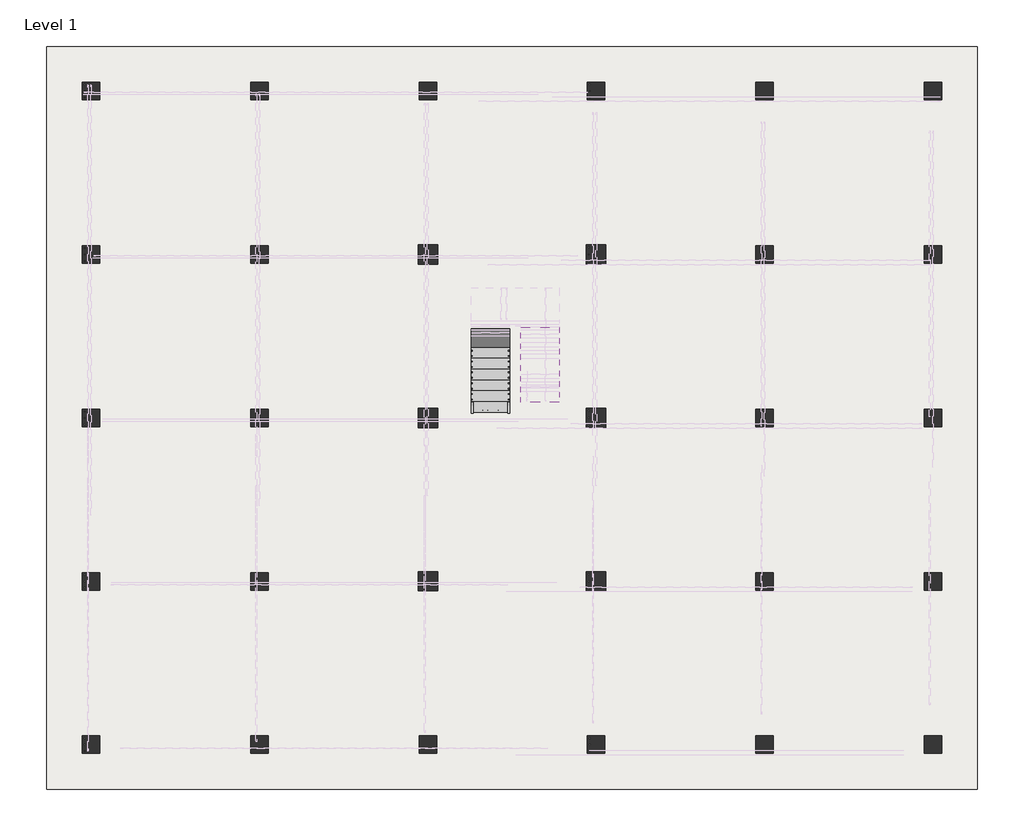
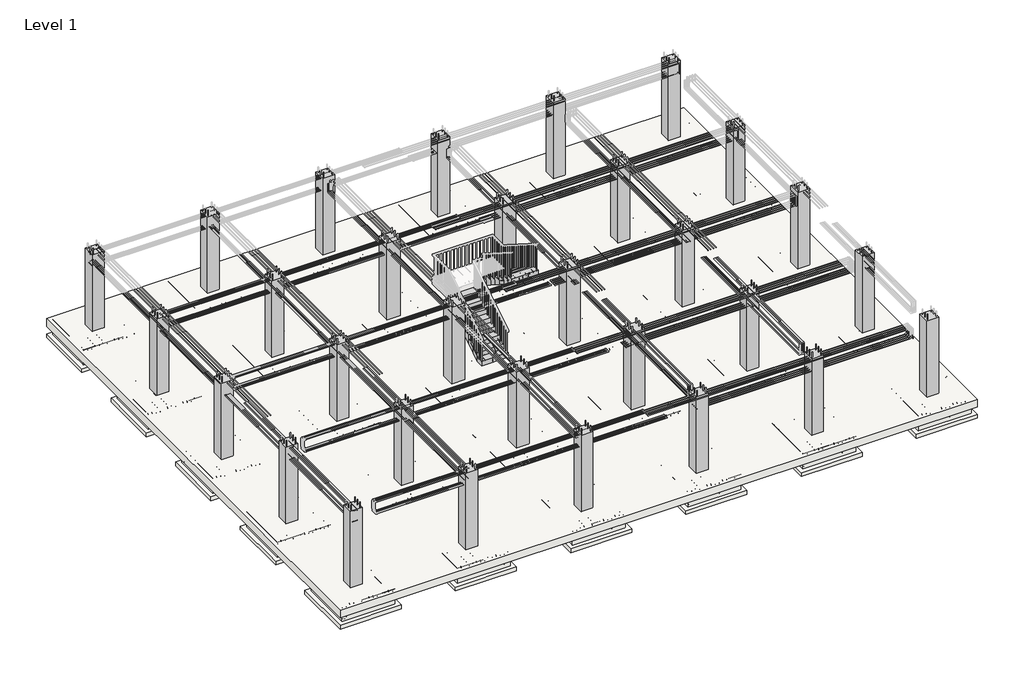
# One storey, part 1 of 17: 31 slabs, 30 columns, 2 stair flights.
"""IFC4 building model written with IfcOpenShell, lengths in millimetres."""

from ifc_helpers import new_model, si_unit, frame, origin, origin_with_axes, place, context, project, spatial, polyline, outline, extrude, faceted_brep, transform, mapped, element, save
from components import m_footing_rectangular_2000x2000x600_e4767d7a, m_footing_rectangular_2200x2200x650_5a9dd948

model = new_model("IFC4")

# Units and contexts
model_context = context("Model", 3, world=origin())
ifc_project = project(units=[si_unit("LENGTHUNIT", "METRE", prefix="MILLI")], contexts=[model_context])

# Site, building, storey
site = spatial("IfcSite", under=ifc_project)
building = spatial("IfcBuilding", under=site)
storey = spatial("IfcBuildingStorey", under=building, Name="Level 1", Elevation=0.0)

# Columns
placement = place(None, origin())
element("IfcColumn", 1, ObjectType="M_Concrete-Rectangular-Column : 450x450", at=placement, inside=storey, context=model_context, shape_type="SweptSolid", body=[
    extrude(outline(polyline([(-12509.3632003, 12560.009457), (-12509.3632003, 12110.009457), (-12959.3632003, 12110.009457), (-12959.3632003, 12560.009457), (-12509.3632003, 12560.009457)])), origin_with_axes(), (0.0, 0.0, 1.0), 3048.0),
])
element("IfcColumn", 2, ObjectType="M_Concrete-Rectangular-Column : 450x450", at=placement, inside=storey, context=model_context, shape_type="SweptSolid", body=[
    extrude(outline(polyline([(-8164.3632003, 12560.009457), (-8164.3632003, 12110.009457), (-8614.3632003, 12110.009457), (-8614.3632003, 12560.009457), (-8164.3632003, 12560.009457)])), origin_with_axes(), (0.0, 0.0, 1.0), 3048.0),
])
element("IfcColumn", 3, ObjectType="M_Concrete-Rectangular-Column : 450x450", at=placement, inside=storey, context=model_context, shape_type="SweptSolid", body=[
    extrude(outline(polyline([(-3819.3632003, 12560.009457), (-3819.3632003, 12110.009457), (-4269.3632003, 12110.009457), (-4269.3632003, 12560.009457), (-3819.3632003, 12560.009457)])), origin_with_axes(), (0.0, 0.0, 1.0), 3048.0),
])
element("IfcColumn", 4, ObjectType="M_Concrete-Rectangular-Column : 450x450", at=placement, inside=storey, context=model_context, shape_type="SweptSolid", body=[
    extrude(outline(polyline([(525.6367997, 12560.009457), (525.6367997, 12110.009457), (75.6367997, 12110.009457), (75.6367997, 12560.009457), (525.6367997, 12560.009457)])), origin_with_axes(), (0.0, 0.0, 1.0), 3048.0),
])
element("IfcColumn", 5, ObjectType="M_Concrete-Rectangular-Column : 450x450", at=placement, inside=storey, context=model_context, shape_type="SweptSolid", body=[
    extrude(outline(polyline([(4870.6367997, 12560.009457), (4870.6367997, 12110.009457), (4420.6367997, 12110.009457), (4420.6367997, 12560.009457), (4870.6367997, 12560.009457)])), origin_with_axes(), (0.0, 0.0, 1.0), 3048.0),
])
element("IfcColumn", 6, ObjectType="M_Concrete-Rectangular-Column : 450x450", at=placement, inside=storey, context=model_context, shape_type="SweptSolid", body=[
    extrude(outline(polyline([(9215.6367997, 12560.009457), (9215.6367997, 12110.009457), (8765.6367997, 12110.009457), (8765.6367997, 12560.009457), (9215.6367997, 12560.009457)])), origin_with_axes(), (0.0, 0.0, 1.0), 3048.0),
])
element("IfcColumn", 7, ObjectType="M_Concrete-Rectangular-Column : 450x450", at=placement, inside=storey, context=model_context, shape_type="SweptSolid", body=[
    extrude(outline(polyline([(-12509.3632003, 8343.009457), (-12509.3632003, 7893.009457), (-12959.3632003, 7893.009457), (-12959.3632003, 8343.009457), (-12509.3632003, 8343.009457)])), origin_with_axes(), (0.0, 0.0, 1.0), 3048.0),
])
element("IfcColumn", 8, ObjectType="M_Concrete-Rectangular-Column : 450x450", at=placement, inside=storey, context=model_context, shape_type="SweptSolid", body=[
    extrude(outline(polyline([(-8164.3632003, 8343.009457), (-8164.3632003, 7893.009457), (-8614.3632003, 7893.009457), (-8614.3632003, 8343.009457), (-8164.3632003, 8343.009457)])), origin_with_axes(), (0.0, 0.0, 1.0), 3048.0),
])
element("IfcColumn", 9, ObjectType="M_Concrete-Rectangular-Column : 450x450", at=placement, inside=storey, context=model_context, shape_type="SweptSolid", body=[
    extrude(outline(polyline([(4870.6367997, 8343.009457), (4870.6367997, 7893.009457), (4420.6367997, 7893.009457), (4420.6367997, 8343.009457), (4870.6367997, 8343.009457)])), origin_with_axes(), (0.0, 0.0, 1.0), 3048.0),
])
element("IfcColumn", 10, ObjectType="M_Concrete-Rectangular-Column : 450x450", at=placement, inside=storey, context=model_context, shape_type="SweptSolid", body=[
    extrude(outline(polyline([(9215.6367997, 8343.009457), (9215.6367997, 7893.009457), (8765.6367997, 7893.009457), (8765.6367997, 8343.009457), (9215.6367997, 8343.009457)])), origin_with_axes(), (0.0, 0.0, 1.0), 3048.0),
])
element("IfcColumn", 11, ObjectType="M_Concrete-Rectangular-Column : 450x450", at=placement, inside=storey, context=model_context, shape_type="SweptSolid", body=[
    extrude(outline(polyline([(-12509.3632003, 4126.009457), (-12509.3632003, 3676.009457), (-12959.3632003, 3676.009457), (-12959.3632003, 4126.009457), (-12509.3632003, 4126.009457)])), origin_with_axes(), (0.0, 0.0, 1.0), 3048.0),
])
element("IfcColumn", 12, ObjectType="M_Concrete-Rectangular-Column : 450x450", at=placement, inside=storey, context=model_context, shape_type="SweptSolid", body=[
    extrude(outline(polyline([(-8164.3632003, 4126.009457), (-8164.3632003, 3676.009457), (-8614.3632003, 3676.009457), (-8614.3632003, 4126.009457), (-8164.3632003, 4126.009457)])), origin_with_axes(), (0.0, 0.0, 1.0), 3048.0),
])
element("IfcColumn", 13, ObjectType="M_Concrete-Rectangular-Column : 450x450", at=placement, inside=storey, context=model_context, shape_type="SweptSolid", body=[
    extrude(outline(polyline([(4870.6367997, 4126.009457), (4870.6367997, 3676.009457), (4420.6367997, 3676.009457), (4420.6367997, 4126.009457), (4870.6367997, 4126.009457)])), origin_with_axes(), (0.0, 0.0, 1.0), 3048.0),
])
element("IfcColumn", 14, ObjectType="M_Concrete-Rectangular-Column : 450x450", at=placement, inside=storey, context=model_context, shape_type="SweptSolid", body=[
    extrude(outline(polyline([(9215.6367997, 4126.009457), (9215.6367997, 3676.009457), (8765.6367997, 3676.009457), (8765.6367997, 4126.009457), (9215.6367997, 4126.009457)])), origin_with_axes(), (0.0, 0.0, 1.0), 3048.0),
])
element("IfcColumn", 15, ObjectType="M_Concrete-Rectangular-Column : 450x450", at=placement, inside=storey, context=model_context, shape_type="SweptSolid", body=[
    extrude(outline(polyline([(-12509.3632003, -90.990543), (-12509.3632003, -540.990543), (-12959.3632003, -540.990543), (-12959.3632003, -90.990543), (-12509.3632003, -90.990543)])), origin_with_axes(), (0.0, 0.0, 1.0), 3048.0),
])
element("IfcColumn", 16, ObjectType="M_Concrete-Rectangular-Column : 450x450", at=placement, inside=storey, context=model_context, shape_type="SweptSolid", body=[
    extrude(outline(polyline([(-8164.3632003, -90.990543), (-8164.3632003, -540.990543), (-8614.3632003, -540.990543), (-8614.3632003, -90.990543), (-8164.3632003, -90.990543)])), origin_with_axes(), (0.0, 0.0, 1.0), 3048.0),
])
element("IfcColumn", 17, ObjectType="M_Concrete-Rectangular-Column : 450x450", at=placement, inside=storey, context=model_context, shape_type="SweptSolid", body=[
    extrude(outline(polyline([(4870.6367997, -90.990543), (4870.6367997, -540.990543), (4420.6367997, -540.990543), (4420.6367997, -90.990543), (4870.6367997, -90.990543)])), origin_with_axes(), (0.0, 0.0, 1.0), 3048.0),
])
element("IfcColumn", 18, ObjectType="M_Concrete-Rectangular-Column : 450x450", at=placement, inside=storey, context=model_context, shape_type="SweptSolid", body=[
    extrude(outline(polyline([(9215.6367997, -90.990543), (9215.6367997, -540.990543), (8765.6367997, -540.990543), (8765.6367997, -90.990543), (9215.6367997, -90.990543)])), origin_with_axes(), (0.0, 0.0, 1.0), 3048.0),
])
element("IfcColumn", 19, ObjectType="M_Concrete-Rectangular-Column : 450x450", at=placement, inside=storey, context=model_context, shape_type="SweptSolid", body=[
    extrude(outline(polyline([(-12509.3632003, -4307.990543), (-12509.3632003, -4757.990543), (-12959.3632003, -4757.990543), (-12959.3632003, -4307.990543), (-12509.3632003, -4307.990543)])), origin_with_axes(), (0.0, 0.0, 1.0), 3048.0),
])
element("IfcColumn", 20, ObjectType="M_Concrete-Rectangular-Column : 450x450", at=placement, inside=storey, context=model_context, shape_type="SweptSolid", body=[
    extrude(outline(polyline([(-8164.3632003, -4307.990543), (-8164.3632003, -4757.990543), (-8614.3632003, -4757.990543), (-8614.3632003, -4307.990543), (-8164.3632003, -4307.990543)])), origin_with_axes(), (0.0, 0.0, 1.0), 3048.0),
])
element("IfcColumn", 21, ObjectType="M_Concrete-Rectangular-Column : 450x450", at=placement, inside=storey, context=model_context, shape_type="SweptSolid", body=[
    extrude(outline(polyline([(-3819.3632003, -4307.990543), (-3819.3632003, -4757.990543), (-4269.3632003, -4757.990543), (-4269.3632003, -4307.990543), (-3819.3632003, -4307.990543)])), origin_with_axes(), (0.0, 0.0, 1.0), 3048.0),
])
element("IfcColumn", 22, ObjectType="M_Concrete-Rectangular-Column : 450x450", at=placement, inside=storey, context=model_context, shape_type="SweptSolid", body=[
    extrude(outline(polyline([(525.6367997, -4307.990543), (525.6367997, -4757.990543), (75.6367997, -4757.990543), (75.6367997, -4307.990543), (525.6367997, -4307.990543)])), origin_with_axes(), (0.0, 0.0, 1.0), 3048.0),
])
element("IfcColumn", 23, ObjectType="M_Concrete-Rectangular-Column : 450x450", at=placement, inside=storey, context=model_context, shape_type="SweptSolid", body=[
    extrude(outline(polyline([(4870.6367997, -4307.990543), (4870.6367997, -4757.990543), (4420.6367997, -4757.990543), (4420.6367997, -4307.990543), (4870.6367997, -4307.990543)])), origin_with_axes(), (0.0, 0.0, 1.0), 3048.0),
])
element("IfcColumn", 24, ObjectType="M_Concrete-Rectangular-Column : 450x450", at=placement, inside=storey, context=model_context, shape_type="SweptSolid", body=[
    extrude(outline(polyline([(9215.6367997, -4307.990543), (9215.6367997, -4757.990543), (8765.6367997, -4757.990543), (8765.6367997, -4307.990543), (9215.6367997, -4307.990543)])), origin_with_axes(), (0.0, 0.0, 1.0), 3048.0),
])
element("IfcColumn", 25, ObjectType="M_Concrete-Rectangular-Column : 500x500", at=placement, inside=storey, context=model_context, shape_type="SweptSolid", body=[
    extrude(outline(polyline([(-3794.3632003, 8368.009457), (-3794.3632003, 7868.009457), (-4294.3632003, 7868.009457), (-4294.3632003, 8368.009457), (-3794.3632003, 8368.009457)])), origin_with_axes(), (0.0, 0.0, 1.0), 3048.0),
])
element("IfcColumn", 26, ObjectType="M_Concrete-Rectangular-Column : 500x500", at=placement, inside=storey, context=model_context, shape_type="SweptSolid", body=[
    extrude(outline(polyline([(550.6367997, 8368.009457), (550.6367997, 7868.009457), (50.6367997, 7868.009457), (50.6367997, 8368.009457), (550.6367997, 8368.009457)])), origin_with_axes(), (0.0, 0.0, 1.0), 3048.0),
])
element("IfcColumn", 27, ObjectType="M_Concrete-Rectangular-Column : 500x500", at=placement, inside=storey, context=model_context, shape_type="SweptSolid", body=[
    extrude(outline(polyline([(550.6367997, 4151.009457), (550.6367997, 3651.009457), (50.6367997, 3651.009457), (50.6367997, 4151.009457), (550.6367997, 4151.009457)])), origin_with_axes(), (0.0, 0.0, 1.0), 3048.0),
])
element("IfcColumn", 28, ObjectType="M_Concrete-Rectangular-Column : 500x500", at=placement, inside=storey, context=model_context, shape_type="SweptSolid", body=[
    extrude(outline(polyline([(-3794.3632003, 4151.009457), (-3794.3632003, 3651.009457), (-4294.3632003, 3651.009457), (-4294.3632003, 4151.009457), (-3794.3632003, 4151.009457)])), origin_with_axes(), (0.0, 0.0, 1.0), 3048.0),
])
element("IfcColumn", 29, ObjectType="M_Concrete-Rectangular-Column : 500x500", at=placement, inside=storey, context=model_context, shape_type="SweptSolid", body=[
    extrude(outline(polyline([(-3794.3632003, -65.990543), (-3794.3632003, -565.990543), (-4294.3632003, -565.990543), (-4294.3632003, -65.990543), (-3794.3632003, -65.990543)])), origin_with_axes(), (0.0, 0.0, 1.0), 3048.0),
])
element("IfcColumn", 30, ObjectType="M_Concrete-Rectangular-Column : 500x500", at=placement, inside=storey, context=model_context, shape_type="SweptSolid", body=[
    extrude(outline(polyline([(550.6367997, -65.990543), (550.6367997, -565.990543), (50.6367997, -565.990543), (50.6367997, -65.990543), (550.6367997, -65.990543)])), origin_with_axes(), (0.0, 0.0, 1.0), 3048.0),
])

# Slabs
element("IfcSlab", 31, ObjectType="Generic 300mm", at=placement, inside=storey, context=model_context, shape_type="SweptSolid", body=[
    extrude(outline(polyline([(10140.6367997, 13485.009457), (10140.6367997, -5682.990543), (-13884.3632003, -5682.990543), (-13884.3632003, 13485.009457), (10140.6367997, 13485.009457)])), frame((0.0, 0.0, -300.0), z_axis=(0.0, 0.0, 1.0), x_axis=(1.0, 0.0, 0.0)), (0.0, 0.0, 1.0), 300.0),
])
m_footing_rectangular_2000x2000x600_shape = m_footing_rectangular_2000x2000x600_e4767d7a(model_context)
element("IfcSlab", 32, ObjectType="M_Footing-Rectangular : 2000x2000x600", at=placement, inside=storey, context=model_context, shape_type="MappedRepresentation", body=[
    mapped(m_footing_rectangular_2000x2000x600_shape, transform((-12734.3632003, 12335.009457, 0.0), x_axis=(1.0, 0.0, 0.0), y_axis=(0.0, 1.0, 0.0), z_axis=(0.0, 0.0, 1.0))),
])
element("IfcSlab", 33, ObjectType="M_Footing-Rectangular : 2000x2000x600", at=placement, inside=storey, context=model_context, shape_type="MappedRepresentation", body=[
    mapped(m_footing_rectangular_2000x2000x600_shape, transform((-8389.3632003, 12335.009457, 0.0), x_axis=(1.0, 0.0, 0.0), y_axis=(0.0, 1.0, 0.0), z_axis=(0.0, 0.0, 1.0))),
])
element("IfcSlab", 34, ObjectType="M_Footing-Rectangular : 2000x2000x600", at=placement, inside=storey, context=model_context, shape_type="MappedRepresentation", body=[
    mapped(m_footing_rectangular_2000x2000x600_shape, transform((-4044.3632003, 12335.009457, 0.0), x_axis=(1.0, 0.0, 0.0), y_axis=(0.0, 1.0, 0.0), z_axis=(0.0, 0.0, 1.0))),
])
element("IfcSlab", 35, ObjectType="M_Footing-Rectangular : 2000x2000x600", at=placement, inside=storey, context=model_context, shape_type="MappedRepresentation", body=[
    mapped(m_footing_rectangular_2000x2000x600_shape, transform((300.6367997, 12335.009457, 0.0), x_axis=(1.0, 0.0, 0.0), y_axis=(0.0, 1.0, 0.0), z_axis=(0.0, 0.0, 1.0))),
])
element("IfcSlab", 36, ObjectType="M_Footing-Rectangular : 2000x2000x600", at=placement, inside=storey, context=model_context, shape_type="MappedRepresentation", body=[
    mapped(m_footing_rectangular_2000x2000x600_shape, transform((4645.6367997, 12335.009457, 0.0), x_axis=(1.0, 0.0, 0.0), y_axis=(0.0, 1.0, 0.0), z_axis=(0.0, 0.0, 1.0))),
])
element("IfcSlab", 37, ObjectType="M_Footing-Rectangular : 2000x2000x600", at=placement, inside=storey, context=model_context, shape_type="MappedRepresentation", body=[
    mapped(m_footing_rectangular_2000x2000x600_shape, transform((8990.6367997, 12335.009457, 0.0), x_axis=(1.0, 0.0, 0.0), y_axis=(0.0, 1.0, 0.0), z_axis=(0.0, 0.0, 1.0))),
])
element("IfcSlab", 38, ObjectType="M_Footing-Rectangular : 2000x2000x600", at=placement, inside=storey, context=model_context, shape_type="MappedRepresentation", body=[
    mapped(m_footing_rectangular_2000x2000x600_shape, transform((-12734.3632003, 8118.009457, 0.0), x_axis=(1.0, 0.0, 0.0), y_axis=(0.0, 1.0, 0.0), z_axis=(0.0, 0.0, 1.0))),
])
element("IfcSlab", 39, ObjectType="M_Footing-Rectangular : 2000x2000x600", at=placement, inside=storey, context=model_context, shape_type="MappedRepresentation", body=[
    mapped(m_footing_rectangular_2000x2000x600_shape, transform((-8389.3632003, 8118.009457, 0.0), x_axis=(1.0, 0.0, 0.0), y_axis=(0.0, 1.0, 0.0), z_axis=(0.0, 0.0, 1.0))),
])
element("IfcSlab", 40, ObjectType="M_Footing-Rectangular : 2000x2000x600", at=placement, inside=storey, context=model_context, shape_type="MappedRepresentation", body=[
    mapped(m_footing_rectangular_2000x2000x600_shape, transform((4645.6367997, 8118.009457, 0.0), x_axis=(1.0, 0.0, 0.0), y_axis=(0.0, 1.0, 0.0), z_axis=(0.0, 0.0, 1.0))),
])
element("IfcSlab", 41, ObjectType="M_Footing-Rectangular : 2000x2000x600", at=placement, inside=storey, context=model_context, shape_type="MappedRepresentation", body=[
    mapped(m_footing_rectangular_2000x2000x600_shape, transform((8990.6367997, 8118.009457, 0.0), x_axis=(1.0, 0.0, 0.0), y_axis=(0.0, 1.0, 0.0), z_axis=(0.0, 0.0, 1.0))),
])
element("IfcSlab", 42, ObjectType="M_Footing-Rectangular : 2000x2000x600", at=placement, inside=storey, context=model_context, shape_type="MappedRepresentation", body=[
    mapped(m_footing_rectangular_2000x2000x600_shape, transform((-12734.3632003, 3901.009457, 0.0), x_axis=(1.0, 0.0, 0.0), y_axis=(0.0, 1.0, 0.0), z_axis=(0.0, 0.0, 1.0))),
])
element("IfcSlab", 43, ObjectType="M_Footing-Rectangular : 2000x2000x600", at=placement, inside=storey, context=model_context, shape_type="MappedRepresentation", body=[
    mapped(m_footing_rectangular_2000x2000x600_shape, transform((-8389.3632003, 3901.009457, 0.0), x_axis=(1.0, 0.0, 0.0), y_axis=(0.0, 1.0, 0.0), z_axis=(0.0, 0.0, 1.0))),
])
element("IfcSlab", 44, ObjectType="M_Footing-Rectangular : 2000x2000x600", at=placement, inside=storey, context=model_context, shape_type="MappedRepresentation", body=[
    mapped(m_footing_rectangular_2000x2000x600_shape, transform((4645.6367997, 3901.009457, 0.0), x_axis=(1.0, 0.0, 0.0), y_axis=(0.0, 1.0, 0.0), z_axis=(0.0, 0.0, 1.0))),
])
element("IfcSlab", 45, ObjectType="M_Footing-Rectangular : 2000x2000x600", at=placement, inside=storey, context=model_context, shape_type="MappedRepresentation", body=[
    mapped(m_footing_rectangular_2000x2000x600_shape, transform((8990.6367997, 3901.009457, 0.0), x_axis=(1.0, 0.0, 0.0), y_axis=(0.0, 1.0, 0.0), z_axis=(0.0, 0.0, 1.0))),
])
element("IfcSlab", 46, ObjectType="M_Footing-Rectangular : 2000x2000x600", at=placement, inside=storey, context=model_context, shape_type="MappedRepresentation", body=[
    mapped(m_footing_rectangular_2000x2000x600_shape, transform((-12734.3632003, -315.990543, 0.0), x_axis=(1.0, 0.0, 0.0), y_axis=(0.0, 1.0, 0.0), z_axis=(0.0, 0.0, 1.0))),
])
element("IfcSlab", 47, ObjectType="M_Footing-Rectangular : 2000x2000x600", at=placement, inside=storey, context=model_context, shape_type="MappedRepresentation", body=[
    mapped(m_footing_rectangular_2000x2000x600_shape, transform((-8389.3632003, -315.990543, 0.0), x_axis=(1.0, 0.0, 0.0), y_axis=(0.0, 1.0, 0.0), z_axis=(0.0, 0.0, 1.0))),
])
element("IfcSlab", 48, ObjectType="M_Footing-Rectangular : 2000x2000x600", at=placement, inside=storey, context=model_context, shape_type="MappedRepresentation", body=[
    mapped(m_footing_rectangular_2000x2000x600_shape, transform((4645.6367997, -315.990543, 0.0), x_axis=(1.0, 0.0, 0.0), y_axis=(0.0, 1.0, 0.0), z_axis=(0.0, 0.0, 1.0))),
])
element("IfcSlab", 49, ObjectType="M_Footing-Rectangular : 2000x2000x600", at=placement, inside=storey, context=model_context, shape_type="MappedRepresentation", body=[
    mapped(m_footing_rectangular_2000x2000x600_shape, transform((8990.6367997, -315.990543, 0.0), x_axis=(1.0, 0.0, 0.0), y_axis=(0.0, 1.0, 0.0), z_axis=(0.0, 0.0, 1.0))),
])
element("IfcSlab", 50, ObjectType="M_Footing-Rectangular : 2000x2000x600", at=placement, inside=storey, context=model_context, shape_type="MappedRepresentation", body=[
    mapped(m_footing_rectangular_2000x2000x600_shape, transform((-12734.3632003, -4532.990543, 0.0), x_axis=(1.0, 0.0, 0.0), y_axis=(0.0, 1.0, 0.0), z_axis=(0.0, 0.0, 1.0))),
])
element("IfcSlab", 51, ObjectType="M_Footing-Rectangular : 2000x2000x600", at=placement, inside=storey, context=model_context, shape_type="MappedRepresentation", body=[
    mapped(m_footing_rectangular_2000x2000x600_shape, transform((-8389.3632003, -4532.990543, 0.0), x_axis=(1.0, 0.0, 0.0), y_axis=(0.0, 1.0, 0.0), z_axis=(0.0, 0.0, 1.0))),
])
element("IfcSlab", 52, ObjectType="M_Footing-Rectangular : 2000x2000x600", at=placement, inside=storey, context=model_context, shape_type="MappedRepresentation", body=[
    mapped(m_footing_rectangular_2000x2000x600_shape, transform((-4044.3632003, -4532.990543, 0.0), x_axis=(1.0, 0.0, 0.0), y_axis=(0.0, 1.0, 0.0), z_axis=(0.0, 0.0, 1.0))),
])
element("IfcSlab", 53, ObjectType="M_Footing-Rectangular : 2000x2000x600", at=placement, inside=storey, context=model_context, shape_type="MappedRepresentation", body=[
    mapped(m_footing_rectangular_2000x2000x600_shape, transform((300.6367997, -4532.990543, 0.0), x_axis=(1.0, 0.0, 0.0), y_axis=(0.0, 1.0, 0.0), z_axis=(0.0, 0.0, 1.0))),
])
element("IfcSlab", 54, ObjectType="M_Footing-Rectangular : 2000x2000x600", at=placement, inside=storey, context=model_context, shape_type="MappedRepresentation", body=[
    mapped(m_footing_rectangular_2000x2000x600_shape, transform((4645.6367997, -4532.990543, 0.0), x_axis=(1.0, 0.0, 0.0), y_axis=(0.0, 1.0, 0.0), z_axis=(0.0, 0.0, 1.0))),
])
element("IfcSlab", 55, ObjectType="M_Footing-Rectangular : 2000x2000x600", at=placement, inside=storey, context=model_context, shape_type="MappedRepresentation", body=[
    mapped(m_footing_rectangular_2000x2000x600_shape, transform((8990.6367997, -4532.990543, 0.0), x_axis=(1.0, 0.0, 0.0), y_axis=(0.0, 1.0, 0.0), z_axis=(0.0, 0.0, 1.0))),
])
m_footing_rectangular_2200x2200x650_shape = m_footing_rectangular_2200x2200x650_5a9dd948(model_context)
element("IfcSlab", 56, ObjectType="M_Footing-Rectangular : 2200x2200x650", at=placement, inside=storey, context=model_context, shape_type="MappedRepresentation", body=[
    mapped(m_footing_rectangular_2200x2200x650_shape, transform((-4044.3632003, 8118.009457, 0.0), x_axis=(1.0, 0.0, 0.0), y_axis=(0.0, 1.0, 0.0), z_axis=(0.0, 0.0, 1.0))),
])
element("IfcSlab", 57, ObjectType="M_Footing-Rectangular : 2200x2200x650", at=placement, inside=storey, context=model_context, shape_type="MappedRepresentation", body=[
    mapped(m_footing_rectangular_2200x2200x650_shape, transform((300.6367997, 8118.009457, 0.0), x_axis=(1.0, 0.0, 0.0), y_axis=(0.0, 1.0, 0.0), z_axis=(0.0, 0.0, 1.0))),
])
element("IfcSlab", 58, ObjectType="M_Footing-Rectangular : 2200x2200x650", at=placement, inside=storey, context=model_context, shape_type="MappedRepresentation", body=[
    mapped(m_footing_rectangular_2200x2200x650_shape, transform((300.6367997, 3901.009457, 0.0), x_axis=(1.0, 0.0, 0.0), y_axis=(0.0, 1.0, 0.0), z_axis=(0.0, 0.0, 1.0))),
])
element("IfcSlab", 59, ObjectType="M_Footing-Rectangular : 2200x2200x650", at=placement, inside=storey, context=model_context, shape_type="MappedRepresentation", body=[
    mapped(m_footing_rectangular_2200x2200x650_shape, transform((-4044.3632003, 3901.009457, 0.0), x_axis=(1.0, 0.0, 0.0), y_axis=(0.0, 1.0, 0.0), z_axis=(0.0, 0.0, 1.0))),
])
element("IfcSlab", 60, ObjectType="M_Footing-Rectangular : 2200x2200x650", at=placement, inside=storey, context=model_context, shape_type="MappedRepresentation", body=[
    mapped(m_footing_rectangular_2200x2200x650_shape, transform((-4044.3632003, -315.990543, 0.0), x_axis=(1.0, 0.0, 0.0), y_axis=(0.0, 1.0, 0.0), z_axis=(0.0, 0.0, 1.0))),
])
element("IfcSlab", 61, ObjectType="M_Footing-Rectangular : 2200x2200x650", at=placement, inside=storey, context=model_context, shape_type="MappedRepresentation", body=[
    mapped(m_footing_rectangular_2200x2200x650_shape, transform((300.6367997, -315.990543, 0.0), x_axis=(1.0, 0.0, 0.0), y_axis=(0.0, 1.0, 0.0), z_axis=(0.0, 0.0, 1.0))),
])

# Stair flights
element("IfcStairFlight", 62, ObjectType="25 mm Nosing", at=placement, inside=storey, context=model_context, shape_type="Brep", body=[
    faceted_brep([(-2927.2746575, 4330.4915698, 179.2941176), (-2927.2746575, 4050.4915698, 179.2941176), (-1927.2746575, 4050.4915698, 179.2941176), (-1927.2746575, 4330.4915698, 179.2941176), (-2927.2746575, 4330.4915698, 1.1770685), (-2927.2746575, 4328.6533658, 0.0), (-2927.2746575, 4050.4915698, 0.0), (-1927.2746575, 4050.4915698, 0.0), (-1927.2746575, 4328.6533658, 0.0), (-1927.2746575, 4330.4915698, 1.1770685), (-2927.2746575, 4610.4915698, 358.5882353), (-2927.2746575, 4330.4915698, 358.5882353), (-1927.2746575, 4330.4915698, 358.5882353), (-1927.2746575, 4610.4915698, 358.5882353), (-2927.2746575, 4610.4915698, 180.4711861), (-1927.2746575, 4610.4915698, 180.4711861), (-2927.2746575, 4890.4915698, 537.8823529), (-2927.2746575, 4610.4915698, 537.8823529), (-1927.2746575, 4610.4915698, 537.8823529), (-1927.2746575, 4890.4915698, 537.8823529), (-2927.2746575, 4890.4915698, 359.7653037), (-1927.2746575, 4890.4915698, 359.7653037), (-2927.2746575, 5170.4915698, 717.1764706), (-2927.2746575, 4890.4915698, 717.1764706), (-1927.2746575, 4890.4915698, 717.1764706), (-1927.2746575, 5170.4915698, 717.1764706), (-2927.2746575, 5170.4915698, 539.0594214), (-1927.2746575, 5170.4915698, 539.0594214), (-2927.2746575, 5450.4915698, 896.4705882), (-2927.2746575, 5170.4915698, 896.4705882), (-1927.2746575, 5170.4915698, 896.4705882), (-1927.2746575, 5450.4915698, 896.4705882), (-2927.2746575, 5450.4915698, 718.353539), (-1927.2746575, 5450.4915698, 718.353539), (-2927.2746575, 5730.4915698, 1075.7647059), (-2927.2746575, 5450.4915698, 1075.7647059), (-1927.2746575, 5450.4915698, 1075.7647059), (-1927.2746575, 5730.4915698, 1075.7647059), (-2927.2746575, 5730.4915698, 897.6476567), (-1927.2746575, 5730.4915698, 897.6476567), (-2927.2746575, 6010.4915698, 1255.0588235), (-2927.2746575, 5730.4915698, 1255.0588235), (-1927.2746575, 5730.4915698, 1255.0588235), (-1927.2746575, 6010.4915698, 1255.0588235), (-2927.2746575, 6010.4915698, 1076.9417743), (-1927.2746575, 6010.4915698, 1076.9417743), (-2927.2746575, 6290.4915698, 1434.3529412), (-2927.2746575, 6265.4915698, 1434.3529412), (-2927.2746575, 6010.4915698, 1434.3529412), (-1927.2746575, 6010.4915698, 1434.3529412), (-1927.2746575, 6265.4915698, 1434.3529412), (-1927.2746575, 6290.4915698, 1434.3529412), (-2927.2746575, 6290.4915698, 1256.235892), (-2927.2746575, 6265.4915698, 1240.2274886), (-1927.2746575, 6290.4915698, 1256.235892), (-1927.2746575, 6290.4915698, 1313.6470588)], [[[0, 1, 2, 3]], [[1, 0, 4, 5, 6]], [[2, 1, 6, 7]], [[3, 2, 7, 8, 9]], [[10, 11, 12, 13]], [[11, 10, 14, 4, 0]], [[0, 3, 12, 11]], [[13, 12, 3, 9, 15]], [[16, 17, 18, 19]], [[17, 16, 20, 14, 10]], [[10, 13, 18, 17]], [[19, 18, 13, 15, 21]], [[22, 23, 24, 25]], [[23, 22, 26, 20, 16]], [[16, 19, 24, 23]], [[25, 24, 19, 21, 27]], [[28, 29, 30, 31]], [[29, 28, 32, 26, 22]], [[22, 25, 30, 29]], [[31, 30, 25, 27, 33]], [[34, 35, 36, 37]], [[35, 34, 38, 32, 28]], [[28, 31, 36, 35]], [[37, 36, 31, 33, 39]], [[40, 41, 42, 43]], [[41, 40, 44, 38, 34]], [[34, 37, 42, 41]], [[43, 42, 37, 39, 45]], [[46, 47, 48, 49, 50, 51]], [[47, 46, 52, 53]], [[40, 43, 49, 48]], [[49, 43, 45, 54, 55, 51, 50]], [[46, 51, 55, 54, 52]], [[7, 6, 5, 8]], [[8, 5, 4, 14, 20, 26, 32, 38, 44, 53, 52, 54, 45, 39, 33, 27, 21, 15, 9]], [[48, 47, 53, 44, 40]]]),
])
element("IfcStairFlight", 63, ObjectType="25 mm Nosing", at=placement, inside=storey, context=model_context, shape_type="Brep", body=[
    faceted_brep([(-647.2746575, 5960.4915698, 1792.9411765), (-647.2746575, 6240.4915698, 1792.9411765), (-1647.2746575, 6240.4915698, 1792.9411765), (-1647.2746575, 5960.4915698, 1792.9411765), (-647.2746575, 5960.4915698, 1614.8241273), (-647.2746575, 6240.4915698, 1435.5300096), (-647.2746575, 6240.4915698, 1613.6470588), (-1647.2746575, 6240.4915698, 1435.5300096), (-1647.2746575, 6240.4915698, 1613.6470588), (-1647.2746575, 5960.4915698, 1614.8241273), (-647.2746575, 5680.4915698, 1972.2352941), (-647.2746575, 5960.4915698, 1972.2352941), (-1647.2746575, 5960.4915698, 1972.2352941), (-1647.2746575, 5680.4915698, 1972.2352941), (-647.2746575, 5680.4915698, 1794.1182449), (-1647.2746575, 5680.4915698, 1794.1182449), (-647.2746575, 5400.4915698, 2151.5294118), (-647.2746575, 5680.4915698, 2151.5294118), (-1647.2746575, 5680.4915698, 2151.5294118), (-1647.2746575, 5400.4915698, 2151.5294118), (-647.2746575, 5400.4915698, 1973.4123626), (-1647.2746575, 5400.4915698, 1973.4123626), (-647.2746575, 5120.4915698, 2330.8235294), (-647.2746575, 5400.4915698, 2330.8235294), (-1647.2746575, 5400.4915698, 2330.8235294), (-1647.2746575, 5120.4915698, 2330.8235294), (-647.2746575, 5120.4915698, 2152.7064802), (-1647.2746575, 5120.4915698, 2152.7064802), (-647.2746575, 4840.4915698, 2510.1176471), (-647.2746575, 5120.4915698, 2510.1176471), (-1647.2746575, 5120.4915698, 2510.1176471), (-1647.2746575, 4840.4915698, 2510.1176471), (-647.2746575, 4840.4915698, 2332.0005979), (-1647.2746575, 4840.4915698, 2332.0005979), (-647.2746575, 4560.4915698, 2689.4117647), (-647.2746575, 4840.4915698, 2689.4117647), (-1647.2746575, 4840.4915698, 2689.4117647), (-1647.2746575, 4560.4915698, 2689.4117647), (-647.2746575, 4560.4915698, 2511.2947155), (-1647.2746575, 4560.4915698, 2511.2947155), (-647.2746575, 4305.4915698, 2868.7058824), (-647.2746575, 4560.4915698, 2868.7058824), (-1647.2746575, 4560.4915698, 2868.7058824), (-1647.2746575, 4305.4915698, 2868.7058824), (-647.2746575, 4305.4915698, 2674.5804298), (-1647.2746575, 4305.4915698, 2674.5804298)], [[[0, 1, 2, 3]], [[1, 0, 4, 5, 6]], [[2, 1, 6, 5, 7, 8]], [[3, 2, 8, 7, 9]], [[10, 11, 12, 13]], [[11, 10, 14, 4, 0]], [[12, 11, 0, 3]], [[13, 12, 3, 9, 15]], [[16, 17, 18, 19]], [[17, 16, 20, 14, 10]], [[18, 17, 10, 13]], [[19, 18, 13, 15, 21]], [[22, 23, 24, 25]], [[23, 22, 26, 20, 16]], [[24, 23, 16, 19]], [[25, 24, 19, 21, 27]], [[28, 29, 30, 31]], [[29, 28, 32, 26, 22]], [[30, 29, 22, 25]], [[31, 30, 25, 27, 33]], [[34, 35, 36, 37]], [[35, 34, 38, 32, 28]], [[36, 35, 28, 31]], [[37, 36, 31, 33, 39]], [[40, 41, 42, 43]], [[41, 40, 44, 38, 34]], [[42, 41, 34, 37]], [[43, 42, 37, 39, 45]], [[40, 43, 45, 44]], [[5, 4, 14, 20, 26, 32, 38, 44, 45, 39, 33, 27, 21, 15, 9, 7]]]),
])

save(model, "model.ifc")

# Revit data of these elements
# Grids (mm)
#   "A": line (-12734.363, -8606.29) -> (-12734.363, 15032.831)
#   "B": line (-8389.363, -8606.29) -> (-8389.363, 15032.831)
#   "C": line (-4044.363, -8606.29) -> (-4044.363, 15032.831)
#   "D": line (300.637, -8606.29) -> (300.637, 15032.831)
#   "E": line (4645.637, -8606.29) -> (4645.637, 15032.831)
#   "F": line (8990.637, -8606.29) -> (8990.637, 15032.831)
#   "1": line (13345.479, -4532.991) -> (-16107.799, -4532.991)
#   "2": line (13345.479, -315.991) -> (-16107.799, -315.991)
#   "3": line (13345.479, 3901.009) -> (-16107.799, 3901.009)
#   "4": line (13345.479, 8118.009) -> (-16107.799, 8118.009)
#   "5": line (13345.479, 12335.009) -> (-16107.799, 12335.009)
# Type "M_Concrete-Rectangular-Column : 450x450"
#   b = 450 mm
#   h = 450 mm
#   Structural Material [instance default] = Concrete, Cast-in-Place gray
# Type "M_Concrete-Rectangular-Column : 500x500"
#   b = 500 mm
#   h = 500 mm
#   Structural Material [instance default] = Concrete, Cast-in-Place gray
# Type "Generic 300mm"
#   Function = 0
#   Layers, outside or top first: 300 mm no material (function 1)
# Type "M_Footing-Rectangular : 2000x2000x600"
#   Width = 2000 mm
#   Length = 2000 mm
#   Foundation Thickness = 600 mm
#   Structural Material [instance default] = Concrete, Cast-in-Place gray
#   Assembly Code = ""
# Type "M_Footing-Rectangular : 2200x2200x650"
#   Width = 2200 mm
#   Length = 2200 mm
#   Foundation Thickness = 650 mm
#   Structural Material [instance default] = Concrete, Cast-in-Place gray
#   Assembly Code = ""
# Elements 1, 2, 3, 4, 5, 6, 7, 8, 9, 10, 11, 12, 13, 14, 15, 16, 17, 18, 19, 20, 21, 22, 23, 24 (IfcColumn, "M_Concrete-Rectangular-Column : 450x450")
#   Comments = ""
#   Structural Material = Concrete, Cast-in-Place gray
#   Phase Created = New Construction
#   Materials on its faces: "Concrete, Cast-in-Place gray"
# Elements 25, 26, 27, 28, 29, 30 (IfcColumn, "M_Concrete-Rectangular-Column : 500x500")
#   Comments = ""
#   Structural Material = Concrete, Cast-in-Place gray
#   Phase Created = New Construction
#   Materials on its faces: "Concrete, Cast-in-Place gray"
# Element 31 (IfcSlab, "Generic 300mm")
#   Height Offset From Level = 0 mm
#   built-in parameter 1001954 = 1
#   Phase Created = New Construction
#   Materials on its faces: "Default Floor"
# Elements 32, 33, 34, 35, 36, 37, 38, 39, 40, 41, 42, 43, 44, 45, 46, 47, 48, 49, 50, 51, 52, 53, 54, 55 (IfcSlab, "M_Footing-Rectangular : 2000x2000x600")
#   Comments = ""
#   Structural Material = Concrete, Cast-in-Place gray
#   Phase Created = New Construction
#   Materials on its faces: "Concrete, Cast-in-Place gray"
# Elements 56, 57, 58, 59, 60, 61 (IfcSlab, "M_Footing-Rectangular : 2200x2200x650")
#   Comments = ""
#   Structural Material = Concrete, Cast-in-Place gray
#   Phase Created = New Construction
#   Materials on its faces: "Concrete, Cast-in-Place gray"
# Elements 62, 63 (IfcStairFlight, "25 mm Nosing")
#   Phase Created = New Construction
#   Materials on its faces: "Concrete, Cast In Situ"
# Materials
#   "Concrete, Cast-in-Place gray": class "Concrete", colour RGB 192 192 192, transparency 0, Description = "Cast-in-place concrete", Cost = 0
#   "Default Floor": colour RGB 127 127 127, transparency 0, Cost = 0
#   "Concrete, Cast In Situ": class "Concrete", colour RGB 192 192 192, transparency 0, Description = "physical material", Cost = 0
